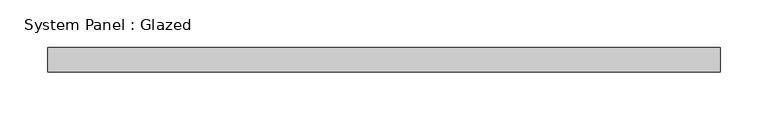
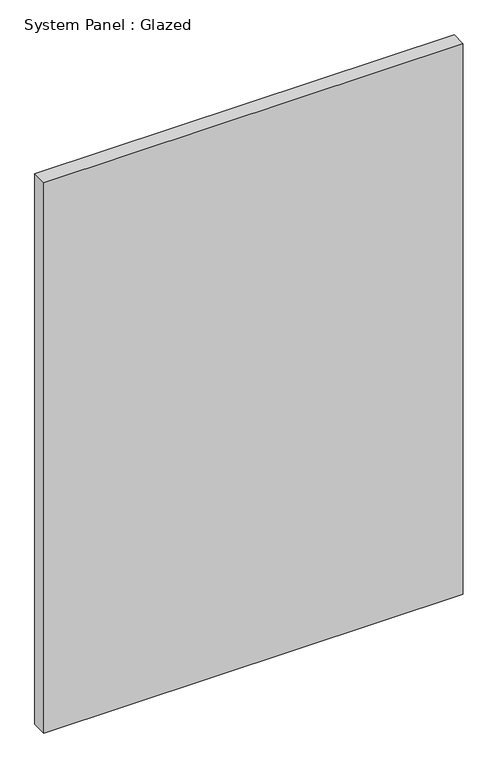
"""IFC4 building model written with IfcOpenShell, lengths in millimetres: plate geometry, System Panel : Glazed."""

from ifc_helpers import new_model, si_unit, origin, origin_with_axes, place, context, project, spatial, polyline, outline, extrude, source, transform, mapped, element, save


def system_panel_glazed_0dd3fac7(model_context):
    return source(origin(), model_context, "Body", "SweptSolid", [
        extrude(outline(polyline([(350.3083333, 19.05), (-350.3083333, 19.05), (-350.3083333, 44.45), (350.3083333, 44.45), (350.3083333, 19.05)])), origin_with_axes(), (0.0, 0.0, 1.0), 971.55),
    ])


if __name__ == "__main__":
    model = new_model("IFC4")
    model_context = context("Model", 3, world=origin())
    ifc_project = project(units=[si_unit("LENGTHUNIT", "METRE", prefix="MILLI")], contexts=[model_context])
    site = spatial("IfcSite", under=ifc_project)
    building = spatial("IfcBuilding", under=site)
    placement = place(None, origin())
    system_panel_glazed_shape = system_panel_glazed_0dd3fac7(model_context)
    element("IfcPlate", 1, ObjectType="System Panel : Glazed", at=placement, inside=building, context=model_context, shape_type="MappedRepresentation", body=[
        mapped(system_panel_glazed_shape, transform((0.0, 0.0, 0.0), x_axis=(1.0, 0.0, 0.0), y_axis=(0.0, 1.0, 0.0), z_axis=(0.0, 0.0, 1.0))),
    ])
    save(model, "model.ifc")

# Revit data of these elements
# Type "System Panel : Glazed"
#   Construction Type Id = "GSP4R"
#   Analytic Construction = "1/8 in Pilkington single glazing"
#   Visual Light Transmittance = 0.9
#   Solar Heat Gain Coefficient = 0.86
#   Heat Transfer Coefficient (U) = 1.18115 BTU/(h·ft²·°F)
# Element 1 (IfcPlate, "System Panel : Glazed")
#   Materials on its faces: "Glass"
# Materials
#   "Glass": class "Glass", colour RGB 0 128 192, transparency 0.75, Description = "Soda Lime Glass", Cost = 0
